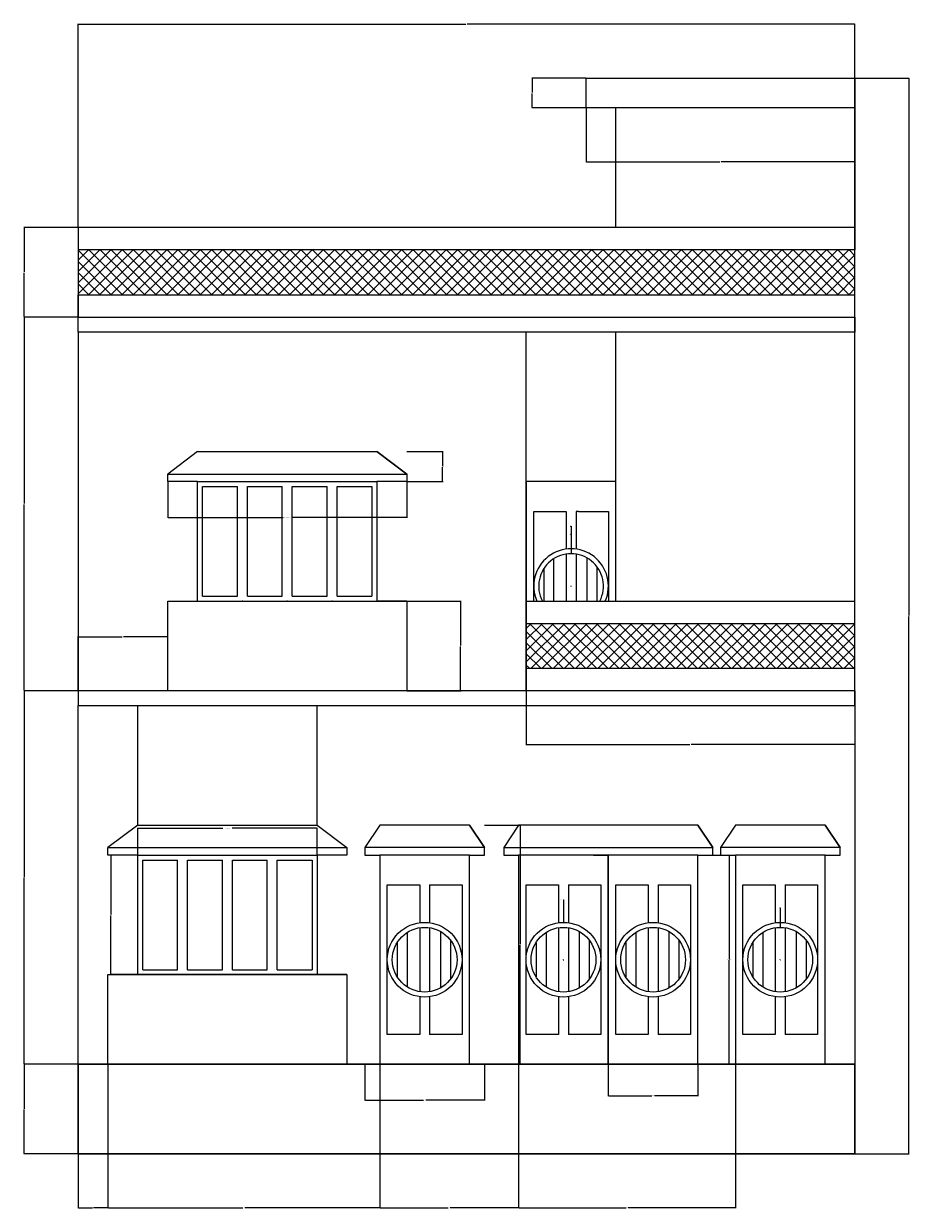
# Model space of a CAD drawing. Units: millimetres. Extents: x 1831 to 2754, y 1517 to 2450.
# Tile 3 of 4: x 1831 to 2186, y 1975 to 2450. Entities that reach past the tile are written whole.
import ezdxf

# ---------------------------------------------------------------- set-up
doc = ezdxf.new("R2010")
doc.units = ezdxf.units.MM
for name, color, linetype, lineweight in [('A-ANNO-DIMS', 2, 'Continuous', 18), ('A-DETL-REFP', 8, 'Continuous', 13), ('A-DOOR', 3, 'Continuous', 25), ('A-ELEV', 7, 'Continuous', 25), ('A-ELEV-BASE', 7, 'Continuous', 30), ('A-ELEV-PATT', 8, 'Continuous', 13), ('A-ELEV-SHAD', 7, 'Continuous', 18), ('A-GLAZ', 4, 'Continuous', 18), ('A-ROOF', 7, 'Continuous', 25)]:
    doc.layers.add(name, color=color, linetype=linetype, lineweight=lineweight)
doc.styles.get("Standard").update_dxf_attribs({"font": 'arial.ttf'})
doc.dimstyles.get("Standard").update_dxf_attribs({"dimtxt": 0.18, "dimasz": 0.18, "dimexe": 0.18, "dimexo": 0.0625, "dimgap": 0.09, "dimtad": 0, "dimtih": 1, "dimtoh": 1, "dimdec": 4, "dimzin": 0, "dimdsep": 46, "dimtxsty": 'Standard', "dimcen": 0.09, "dimadec": 0, "dimazin": 0, "dimtfac": 1, "dimtdec": 4, "dimtofl": 0, "dimtmove": 0, "dimatfit": 3, "dimfxl": 1, "dimtolj": 1, "dimtzin": 0, "dimarcsym": 0})

# ---------------------------------------------------------------- blocks, each defined once
blk = doc.blocks.new('DOOR-ELEV-SINGLE-HOODED')
for p, q in [((6, 96), (0, 87)), ((6, 96), (0, 87)), ((42, 96), (6, 96)), ((42, 96), (6, 96)), ((42, 96), (48, 87)), ((48, 87), (42, 96)), ((42, 96), (48, 87)), ((48, 87), (42, 96)), ((48, 87), (0, 87)), ((0, 87), (0, 84)), ((48, 87), (0, 87)), ((48, 84), (48, 87)), ((0, 84), (6, 84)), ((42, 84), (6, 84)), ((6, 84), (6, 0)), ((42, 84), (6, 84)), ((6, 84), (6, 0)), ((42, 0), (42, 84)), ((42, 84), (48, 84)), ((42, 0), (42, 84)), ((42, 84), (48, 84)), ((9, 72), (21, 72)), ((9, 12), (9, 72)), ((9, 72), (21, 72)), ((9, 12), (9, 72)), ((21, 72), (22, 72)), ((21, 72), (22, 72)), ((22, 72), (22, 56.87)), ((22, 72), (22, 56.87)), ((26, 72), (26, 56.87)), ((26, 72), (27, 72)), ((26, 72), (26, 56.87)), ((26, 72), (27, 72)), ((27, 72), (39, 72)), ((27, 72), (39, 72)), ((39, 72), (39, 12)), ((39, 72), (39, 12)), ((17, 52.95), (17, 31.05)), ((17, 52.95), (17, 31.05)), ((22, 54.85), (22, 29.15)), ((22, 54.85), (22, 29.15)), ((26, 54.85), (26, 29.15)), ((26, 54.85), (26, 29.15)), ((30.5, 30.74), (30.5, 53.26)), ((30.5, 30.74), (30.5, 53.26)), ((30.5, 30.74), (30.5, 53.26)), ((30.5, 30.74), (30.5, 53.26)), ((13, 48.93), (13, 35.07)), ((13, 48.93), (13, 35.07)), ((34.5, 34.34), (34.5, 49.66)), ((34.5, 34.34), (34.5, 49.66)), ((22, 27.13), (22, 12)), ((22, 27.13), (22, 12)), ((26, 27.13), (26, 12)), ((26, 27.13), (26, 12)), ((22, 12), (9, 12)), ((22, 12), (9, 12)), ((39, 12), (26, 12)), ((39, 12), (26, 12)), ((6, 0), (42, 0))]:
    blk.add_line(p, q)
for radius in [15, 15, 13, 13]:
    blk.add_circle((24, 42), radius)
blk = doc.blocks.new('DOOR-ELEV-ORNAMENTAL-LEAF')
for p, q in [((36, 84), (0, 84)), ((0, 84), (0, 0)), ((36, 0), (36, 84)), ((3, 72), (15, 72)), ((3, 12), (3, 72)), ((15, 72), (16, 72)), ((16, 72), (16, 56.87)), ((20, 72), (20, 56.87)), ((20, 72), (21, 72)), ((21, 72), (33, 72)), ((33, 72), (33, 12)), ((11, 52.95), (11, 31.05)), ((16, 54.85), (16, 29.15)), ((20, 54.85), (20, 29.15)), ((24.5, 30.74), (24.5, 53.26)), ((24.5, 30.74), (24.5, 53.26)), ((7, 48.93), (7, 35.07)), ((28.5, 34.34), (28.5, 49.66)), ((16, 27.13), (16, 12)), ((20, 27.13), (20, 12)), ((16, 12), (3, 12)), ((33, 12), (20, 12)), ((0, 0), (36, 0))]:
    blk.add_line(p, q)
for radius in [15, 13]:
    blk.add_circle((18, 42), radius)
blk = doc.blocks.new('WINDOW-ELEV-FOUR-LIGHT')
for p, q in [((0, 0), (0, 48)), ((0, 48), (72, 48)), ((72, 48), (72, 0)), ((2, 46), (16, 46)), ((2, 2), (2, 46)), ((16, 2), (16, 46)), ((20, 2), (20, 46)), ((20, 46), (34, 46)), ((34, 2), (34, 46)), ((38, 2), (38, 46)), ((38, 46), (52, 46)), ((52, 2), (52, 46)), ((56, 2), (56, 46)), ((56, 46), (70, 46)), ((70, 46), (70, 2)), ((0, 0), (72, 0)), ((2, 2), (16, 2)), ((20, 2), (34, 2)), ((38, 2), (52, 2)), ((56, 2), (70, 2))]:
    blk.add_line(p, q)
blk = doc.blocks.new('CANOPY-ELEV-WINDOW')
for p, q in [((12, 12), (0, 3)), ((12, 12), (84, 12)), ((84, 12), (96, 3)), ((0, 0), (0, 3)), ((0, 3), (96, 3)), ((12, 0), (0, 0)), ((96, 0), (84, 0)), ((96, 3), (96, 0))]:
    blk.add_line(p, q)
blk = doc.blocks.new('*D14')
at = {"layer": 'A-ANNO-DIMS', "color": 0, "lineweight": -2, "transparency": 16777216}
for p, q in [((2015.67, 2128.5), (2030.19, 2128.5)), ((2030.01, 2128.32), (2030.01, 2080.68)), ((2030.01, 2032.68), (2030.01, 2080.31)), ((2015.67, 2032.5), (2030.19, 2032.5))]:
    blk.add_line(p, q, dxfattribs=at)
at = {"layer": 'A-ANNO-DIMS', "color": 0, "transparency": 16777216}
for points in [[(2029.98, 2128.32), (2030.04, 2128.32), (2030.01, 2128.5)], [(2029.98, 2032.68), (2030.04, 2032.68), (2030.01, 2032.5)]]:
    blk.add_solid(points, dxfattribs=at)
at = {"layer": 'Defpoints', "color": 0, "transparency": 16777216}
for p in [(2015.61, 2128.5), (2030.01, 2128.5), (2015.61, 2032.5)]:
    blk.add_point(p, dxfattribs=at)
at = {"layer": 'A-ANNO-DIMS', "color": 0, "transparency": 16777216, "insert": (2030.01, 2080.5), "char_height": 0.18, "attachment_point": 5}
blk.add_mtext('\\A1;HOODED ENTRY 96 TYP.', dxfattribs=at)
blk = doc.blocks.new('*D15')
at = {"layer": 'A-ANNO-DIMS', "color": 0, "lineweight": -2, "transparency": 16777216}
for p, q in [((1967.61, 2032.43), (1967.61, 2017.92)), ((2015.61, 2032.43), (2015.61, 2017.92)), ((1967.79, 2018.1), (1991.08, 2018.1)), ((2015.43, 2018.1), (1992.14, 2018.1))]:
    blk.add_line(p, q, dxfattribs=at)
at = {"layer": 'A-ANNO-DIMS', "color": 0, "transparency": 16777216}
for points in [[(1967.79, 2018.13), (1967.79, 2018.07), (1967.61, 2018.1)], [(2015.43, 2018.13), (2015.43, 2018.07), (2015.61, 2018.1)]]:
    blk.add_solid(points, dxfattribs=at)
at = {"layer": 'Defpoints', "color": 0, "transparency": 16777216}
for p in [(1967.61, 2032.5), (2015.61, 2032.5), (2015.61, 2018.1)]:
    blk.add_point(p, dxfattribs=at)
at = {"layer": 'A-ANNO-DIMS', "color": 0, "transparency": 16777216, "insert": (1991.61, 2018.1), "char_height": 0.18, "attachment_point": 5}
blk.add_mtext('\\A1;48 TYP.', dxfattribs=at)
blk = doc.blocks.new('*D16')
at = {"layer": 'A-ANNO-DIMS', "color": 0, "lineweight": -2, "transparency": 16777216}
for p, q in [((2101.41, 2116.5), (2114.13, 2116.5)), ((2113.95, 2116.32), (2113.95, 2074.68)), ((2113.95, 2032.68), (2113.95, 2074.31)), ((2101.41, 2032.5), (2114.13, 2032.5))]:
    blk.add_line(p, q, dxfattribs=at)
at = {"layer": 'A-ANNO-DIMS', "color": 0, "transparency": 16777216}
for points in [[(2113.92, 2116.32), (2113.98, 2116.32), (2113.95, 2116.5)], [(2113.92, 2032.68), (2113.98, 2032.68), (2113.95, 2032.5)]]:
    blk.add_solid(points, dxfattribs=at)
at = {"layer": 'Defpoints', "color": 0, "transparency": 16777216}
for p in [(2101.35, 2116.5), (2113.95, 2116.5), (2101.35, 2032.5)]:
    blk.add_point(p, dxfattribs=at)
at = {"layer": 'A-ANNO-DIMS', "color": 0, "transparency": 16777216, "insert": (2113.95, 2074.5), "char_height": 0.18, "attachment_point": 5}
blk.add_mtext('\\A1;GATE LEAF 84 TYP.', dxfattribs=at)
blk = doc.blocks.new('*D17')
at = {"layer": 'A-ANNO-DIMS', "color": 0, "lineweight": -2, "transparency": 16777216}
for p, q in [((2065.35, 2032.43), (2065.35, 2019.72)), ((2101.35, 2032.43), (2101.35, 2019.72)), ((2065.53, 2019.9), (2082.82, 2019.9)), ((2101.17, 2019.9), (2083.88, 2019.9))]:
    blk.add_line(p, q, dxfattribs=at)
at = {"layer": 'A-ANNO-DIMS', "color": 0, "transparency": 16777216}
for points in [[(2065.53, 2019.93), (2065.53, 2019.87), (2065.35, 2019.9)], [(2101.17, 2019.93), (2101.17, 2019.87), (2101.35, 2019.9)]]:
    blk.add_solid(points, dxfattribs=at)
at = {"layer": 'Defpoints', "color": 0, "transparency": 16777216}
for p in [(2065.35, 2032.5), (2101.35, 2032.5), (2101.35, 2019.9)]:
    blk.add_point(p, dxfattribs=at)
at = {"layer": 'A-ANNO-DIMS', "color": 0, "transparency": 16777216, "insert": (2083.35, 2019.9), "char_height": 0.18, "attachment_point": 5}
blk.add_mtext('\\A1;36 TYP.', dxfattribs=at)
blk = doc.blocks.new('*D18')
at = {"layer": 'A-ANNO-DIMS', "color": 0, "lineweight": -2, "transparency": 16777216}
for p, q in [((1876.41, 2116.56), (1876.41, 2127.48)), ((1876.59, 2127.3), (1910.5, 2127.3)), ((1948.23, 2127.3), (1914.32, 2127.3)), ((1948.41, 2116.56), (1948.41, 2127.48))]:
    blk.add_line(p, q, dxfattribs=at)
at = {"layer": 'A-ANNO-DIMS', "color": 0, "transparency": 16777216}
for points in [[(1876.59, 2127.33), (1876.59, 2127.27), (1876.41, 2127.3)], [(1948.23, 2127.33), (1948.23, 2127.27), (1948.41, 2127.3)]]:
    blk.add_solid(points, dxfattribs=at)
at = {"layer": 'Defpoints', "color": 0, "transparency": 16777216}
for p in [(1948.41, 2127.3), (1876.41, 2116.5), (1948.41, 2116.5)]:
    blk.add_point(p, dxfattribs=at)
at = {"layer": 'A-ANNO-DIMS', "color": 0, "transparency": 16777216, "insert": (1912.41, 2127.3), "char_height": 0.18, "attachment_point": 5}
blk.add_mtext('\\A1;FOUR-LIGHT WINDOW 72 TYP.', dxfattribs=at)
blk = doc.blocks.new('*D19')
at = {"layer": 'A-ANNO-DIMS', "color": 0, "lineweight": -2, "transparency": 16777216}
for p, q in [((1876.35, 2116.5), (1865.43, 2116.5)), ((1865.61, 2116.32), (1865.61, 2092.68)), ((1865.61, 2068.68), (1865.61, 2092.31)), ((1876.35, 2068.5), (1865.43, 2068.5))]:
    blk.add_line(p, q, dxfattribs=at)
at = {"layer": 'A-ANNO-DIMS', "color": 0, "transparency": 16777216}
for points in [[(1865.58, 2116.32), (1865.64, 2116.32), (1865.61, 2116.5)], [(1865.58, 2068.68), (1865.64, 2068.68), (1865.61, 2068.5)]]:
    blk.add_solid(points, dxfattribs=at)
at = {"layer": 'Defpoints', "color": 0, "transparency": 16777216}
for p in [(1865.61, 2116.5), (1876.41, 2116.5), (1876.41, 2068.5)]:
    blk.add_point(p, dxfattribs=at)
at = {"layer": 'A-ANNO-DIMS', "color": 0, "transparency": 16777216, "insert": (1865.61, 2092.5), "char_height": 0.18, "attachment_point": 5}
blk.add_mtext('\\A1;48 TYP.', dxfattribs=at)
blk = doc.blocks.new('*D20')
at = {"layer": 'A-ANNO-DIMS', "color": 0, "lineweight": -2, "transparency": 16777216}
for p, q in [((1888.41, 2266.43), (1888.41, 2251.92)), ((1984.41, 2266.43), (1984.41, 2251.92)), ((1888.59, 2252.1), (1934.72, 2252.1)), ((1984.23, 2252.1), (1938.09, 2252.1))]:
    blk.add_line(p, q, dxfattribs=at)
at = {"layer": 'A-ANNO-DIMS', "color": 0, "transparency": 16777216}
for points in [[(1888.59, 2252.13), (1888.59, 2252.07), (1888.41, 2252.1)], [(1984.23, 2252.13), (1984.23, 2252.07), (1984.41, 2252.1)]]:
    blk.add_solid(points, dxfattribs=at)
at = {"layer": 'Defpoints', "color": 0, "transparency": 16777216}
for p in [(1888.41, 2266.5), (1984.41, 2266.5), (1984.41, 2252.1)]:
    blk.add_point(p, dxfattribs=at)
at = {"layer": 'A-ANNO-DIMS', "color": 0, "transparency": 16777216, "insert": (1936.41, 2252.1), "char_height": 0.18, "attachment_point": 5}
blk.add_mtext('\\A1;WINDOW CANOPY 96 TYP.', dxfattribs=at)
blk = doc.blocks.new('*D21')
at = {"layer": 'A-ANNO-DIMS', "color": 0, "lineweight": -2, "transparency": 16777216}
for p, q in [((1984.47, 2278.5), (1998.99, 2278.5)), ((1998.81, 2278.32), (1998.81, 2272.68)), ((1998.81, 2266.68), (1998.81, 2272.31)), ((1984.47, 2266.5), (1998.99, 2266.5))]:
    blk.add_line(p, q, dxfattribs=at)
at = {"layer": 'A-ANNO-DIMS', "color": 0, "transparency": 16777216}
for points in [[(1998.78, 2278.32), (1998.84, 2278.32), (1998.81, 2278.5)], [(1998.78, 2266.68), (1998.84, 2266.68), (1998.81, 2266.5)]]:
    blk.add_solid(points, dxfattribs=at)
at = {"layer": 'Defpoints', "color": 0, "transparency": 16777216}
for p in [(1984.41, 2278.5), (1998.81, 2278.5), (1984.41, 2266.5)]:
    blk.add_point(p, dxfattribs=at)
at = {"layer": 'A-ANNO-DIMS', "color": 0, "transparency": 16777216, "insert": (1998.81, 2272.5), "char_height": 0.18, "attachment_point": 5}
blk.add_mtext('\\A1;12 TYP.', dxfattribs=at)
blk = doc.blocks.new('*D45')
at = {"layer": 'A-ANNO-DIMS', "color": 0, "lineweight": -2, "transparency": 16777216}
for p, q in [((1852.41, 2368.56), (1852.41, 2450.31)), ((1852.59, 2450.13), (2008.12, 2450.13)), ((2164.23, 2450.13), (2008.7, 2450.13)), ((2164.41, 2428.56), (2164.41, 2450.31))]:
    blk.add_line(p, q, dxfattribs=at)
at = {"layer": 'A-ANNO-DIMS', "color": 0, "transparency": 16777216}
for points in [[(1852.59, 2450.16), (1852.59, 2450.1), (1852.41, 2450.13)], [(2164.23, 2450.16), (2164.23, 2450.1), (2164.41, 2450.13)]]:
    blk.add_solid(points, dxfattribs=at)
at = {"layer": 'Defpoints', "color": 0, "transparency": 16777216}
for p in [(2164.41, 2450.13), (2164.41, 2428.5), (1852.41, 2368.5)]:
    blk.add_point(p, dxfattribs=at)
at = {"layer": 'A-ANNO-DIMS', "color": 0, "transparency": 16777216, "insert": (2008.41, 2450.13), "char_height": 0.18, "attachment_point": 5}
blk.add_mtext('\\A1;312', dxfattribs=at)
blk = doc.blocks.new('*D46')
at = {"layer": 'A-ANNO-DIMS', "color": 0, "lineweight": -2, "transparency": 16777216}
for p, q in [((2164.47, 2428.5), (2186.22, 2428.5)), ((2186.04, 2428.32), (2186.04, 2212.68)), ((2186.04, 1996.68), (2186.04, 2212.31)), ((2164.47, 1996.5), (2186.22, 1996.5))]:
    blk.add_line(p, q, dxfattribs=at)
at = {"layer": 'A-ANNO-DIMS', "color": 0, "transparency": 16777216}
for points in [[(2186.01, 2428.32), (2186.07, 2428.32), (2186.04, 2428.5)], [(2186.01, 1996.68), (2186.07, 1996.68), (2186.04, 1996.5)]]:
    blk.add_solid(points, dxfattribs=at)
at = {"layer": 'Defpoints', "color": 0, "transparency": 16777216}
for p in [(2164.41, 2428.5), (2186.04, 2428.5), (2164.41, 1996.5)]:
    blk.add_point(p, dxfattribs=at)
at = {"layer": 'A-ANNO-DIMS', "color": 0, "transparency": 16777216, "insert": (2186.04, 2212.5), "char_height": 0.18, "attachment_point": 5}
blk.add_mtext('\\A1;432', dxfattribs=at)
blk = doc.blocks.new('*D47')
at = {"layer": 'A-ANNO-DIMS', "color": 0, "lineweight": -2, "transparency": 16777216}
for p, q in [((1852.35, 2032.5), (1830.6, 2032.5)), ((1830.78, 2032.32), (1830.78, 2014.68)), ((1830.78, 1996.68), (1830.78, 2014.31)), ((1852.35, 1996.5), (1830.6, 1996.5))]:
    blk.add_line(p, q, dxfattribs=at)
at = {"layer": 'A-ANNO-DIMS', "color": 0, "transparency": 16777216}
for points in [[(1830.75, 2032.32), (1830.81, 2032.32), (1830.78, 2032.5)], [(1830.75, 1996.68), (1830.81, 1996.68), (1830.78, 1996.5)]]:
    blk.add_solid(points, dxfattribs=at)
at = {"layer": 'Defpoints', "color": 0, "transparency": 16777216}
for p in [(1830.78, 2032.5), (1852.41, 2032.5), (1852.41, 1996.5)]:
    blk.add_point(p, dxfattribs=at)
at = {"layer": 'A-ANNO-DIMS', "color": 0, "transparency": 16777216, "insert": (1830.78, 2014.5), "char_height": 0.18, "attachment_point": 5}
blk.add_mtext('\\A1;36', dxfattribs=at)
blk = doc.blocks.new('*D48')
at = {"layer": 'A-ANNO-DIMS', "color": 0, "lineweight": -2, "transparency": 16777216}
for p, q in [((1852.35, 2182.5), (1830.6, 2182.5)), ((1830.78, 2182.32), (1830.78, 2107.68)), ((1830.78, 2032.68), (1830.78, 2107.31)), ((1852.35, 2032.5), (1830.6, 2032.5))]:
    blk.add_line(p, q, dxfattribs=at)
at = {"layer": 'A-ANNO-DIMS', "color": 0, "transparency": 16777216}
for points in [[(1830.75, 2182.32), (1830.81, 2182.32), (1830.78, 2182.5)], [(1830.75, 2032.68), (1830.81, 2032.68), (1830.78, 2032.5)]]:
    blk.add_solid(points, dxfattribs=at)
at = {"layer": 'Defpoints', "color": 0, "transparency": 16777216}
for p in [(1830.78, 2182.5), (1852.41, 2182.5), (1852.41, 2032.5)]:
    blk.add_point(p, dxfattribs=at)
at = {"layer": 'A-ANNO-DIMS', "color": 0, "transparency": 16777216, "insert": (1830.78, 2107.5), "char_height": 0.18, "attachment_point": 5}
blk.add_mtext('\\A1;150', dxfattribs=at)
blk = doc.blocks.new('*D49')
at = {"layer": 'A-ANNO-DIMS', "color": 0, "lineweight": -2, "transparency": 16777216}
for p, q in [((1852.35, 2332.5), (1830.6, 2332.5)), ((1830.78, 2332.32), (1830.78, 2257.68)), ((1830.78, 2182.68), (1830.78, 2257.31)), ((1852.35, 2182.5), (1830.6, 2182.5))]:
    blk.add_line(p, q, dxfattribs=at)
at = {"layer": 'A-ANNO-DIMS', "color": 0, "transparency": 16777216}
for points in [[(1830.75, 2332.32), (1830.81, 2332.32), (1830.78, 2332.5)], [(1830.75, 2182.68), (1830.81, 2182.68), (1830.78, 2182.5)]]:
    blk.add_solid(points, dxfattribs=at)
at = {"layer": 'Defpoints', "color": 0, "transparency": 16777216}
for p in [(1830.78, 2332.5), (1852.41, 2332.5), (1852.41, 2182.5)]:
    blk.add_point(p, dxfattribs=at)
at = {"layer": 'A-ANNO-DIMS', "color": 0, "transparency": 16777216, "insert": (1830.78, 2257.5), "char_height": 0.18, "attachment_point": 5}
blk.add_mtext('\\A1;150', dxfattribs=at)
blk = doc.blocks.new('*D50')
at = {"layer": 'A-ANNO-DIMS', "color": 0, "lineweight": -2, "transparency": 16777216}
for p, q in [((1852.35, 2368.5), (1830.6, 2368.5)), ((1830.78, 2368.32), (1830.78, 2350.68)), ((1830.78, 2332.68), (1830.78, 2350.31)), ((1852.35, 2332.5), (1830.6, 2332.5))]:
    blk.add_line(p, q, dxfattribs=at)
at = {"layer": 'A-ANNO-DIMS', "color": 0, "transparency": 16777216}
for points in [[(1830.75, 2368.32), (1830.81, 2368.32), (1830.78, 2368.5)], [(1830.75, 2332.68), (1830.81, 2332.68), (1830.78, 2332.5)]]:
    blk.add_solid(points, dxfattribs=at)
at = {"layer": 'Defpoints', "color": 0, "transparency": 16777216}
for p in [(1830.78, 2368.5), (1852.41, 2368.5), (1852.41, 2332.5)]:
    blk.add_point(p, dxfattribs=at)
at = {"layer": 'A-ANNO-DIMS', "color": 0, "transparency": 16777216, "insert": (1830.78, 2350.5), "char_height": 0.18, "attachment_point": 5}
blk.add_mtext('\\A1;36', dxfattribs=at)
blk = doc.blocks.new('*D51')
at = {"layer": 'A-ANNO-DIMS', "color": 0, "lineweight": -2, "transparency": 16777216}
for p, q in [((2056.41, 2416.43), (2056.41, 2394.69)), ((2164.41, 2416.43), (2164.41, 2394.69)), ((2056.59, 2394.87), (2110.13, 2394.87)), ((2164.23, 2394.87), (2110.69, 2394.87))]:
    blk.add_line(p, q, dxfattribs=at)
at = {"layer": 'A-ANNO-DIMS', "color": 0, "transparency": 16777216}
for points in [[(2056.59, 2394.9), (2056.59, 2394.84), (2056.41, 2394.87)], [(2164.23, 2394.9), (2164.23, 2394.84), (2164.41, 2394.87)]]:
    blk.add_solid(points, dxfattribs=at)
at = {"layer": 'Defpoints', "color": 0, "transparency": 16777216}
for p in [(2056.41, 2416.5), (2164.41, 2416.5), (2056.41, 2394.87)]:
    blk.add_point(p, dxfattribs=at)
at = {"layer": 'A-ANNO-DIMS', "color": 0, "transparency": 16777216, "insert": (2110.41, 2394.87), "char_height": 0.18, "attachment_point": 5}
blk.add_mtext('\\A1;108', dxfattribs=at)
blk = doc.blocks.new('*D52')
at = {"layer": 'A-ANNO-DIMS', "color": 0, "lineweight": -2, "transparency": 16777216}
for p, q in [((2056.35, 2428.5), (2034.6, 2428.5)), ((2034.78, 2428.32), (2034.78, 2422.68)), ((2034.78, 2416.68), (2034.78, 2422.31)), ((2056.35, 2416.5), (2034.6, 2416.5))]:
    blk.add_line(p, q, dxfattribs=at)
at = {"layer": 'A-ANNO-DIMS', "color": 0, "transparency": 16777216}
for points in [[(2034.75, 2428.32), (2034.81, 2428.32), (2034.78, 2428.5)], [(2034.75, 2416.68), (2034.81, 2416.68), (2034.78, 2416.5)]]:
    blk.add_solid(points, dxfattribs=at)
at = {"layer": 'Defpoints', "color": 0, "transparency": 16777216}
for p in [(2034.78, 2428.5), (2056.41, 2428.5), (2056.41, 2416.5)]:
    blk.add_point(p, dxfattribs=at)
at = {"layer": 'A-ANNO-DIMS', "color": 0, "transparency": 16777216, "insert": (2034.78, 2422.5), "char_height": 0.18, "attachment_point": 5}
blk.add_mtext('\\A1;12', dxfattribs=at)
blk = doc.blocks.new('*D53')
at = {"layer": 'A-ANNO-DIMS', "color": 0, "lineweight": -2, "transparency": 16777216}
for p, q in [((2032.41, 2182.43), (2032.41, 2160.69)), ((2164.41, 2182.43), (2164.41, 2160.69)), ((2032.59, 2160.87), (2098.13, 2160.87)), ((2164.23, 2160.87), (2098.69, 2160.87))]:
    blk.add_line(p, q, dxfattribs=at)
at = {"layer": 'A-ANNO-DIMS', "color": 0, "transparency": 16777216}
for points in [[(2032.59, 2160.9), (2032.59, 2160.84), (2032.41, 2160.87)], [(2164.23, 2160.9), (2164.23, 2160.84), (2164.41, 2160.87)]]:
    blk.add_solid(points, dxfattribs=at)
at = {"layer": 'Defpoints', "color": 0, "transparency": 16777216}
for p in [(2032.41, 2182.5), (2164.41, 2182.5), (2032.41, 2160.87)]:
    blk.add_point(p, dxfattribs=at)
at = {"layer": 'A-ANNO-DIMS', "color": 0, "transparency": 16777216, "insert": (2098.41, 2160.87), "char_height": 0.18, "attachment_point": 5}
blk.add_mtext('\\A1;132', dxfattribs=at)
blk = doc.blocks.new('*D54')
at = {"layer": 'A-ANNO-DIMS', "color": 0, "lineweight": -2, "transparency": 16777216}
for p, q in [((1984.47, 2218.5), (2006.22, 2218.5)), ((2006.04, 2218.32), (2006.04, 2200.68)), ((2006.04, 2182.68), (2006.04, 2200.31)), ((1984.47, 2182.5), (2006.22, 2182.5))]:
    blk.add_line(p, q, dxfattribs=at)
at = {"layer": 'A-ANNO-DIMS', "color": 0, "transparency": 16777216}
for points in [[(2006.01, 2218.32), (2006.07, 2218.32), (2006.04, 2218.5)], [(2006.01, 2182.68), (2006.07, 2182.68), (2006.04, 2182.5)]]:
    blk.add_solid(points, dxfattribs=at)
at = {"layer": 'Defpoints', "color": 0, "transparency": 16777216}
for p in [(1984.41, 2218.5), (1984.41, 2182.5), (2006.04, 2182.5)]:
    blk.add_point(p, dxfattribs=at)
at = {"layer": 'A-ANNO-DIMS', "color": 0, "transparency": 16777216, "insert": (2006.04, 2200.5), "char_height": 0.18, "attachment_point": 5}
blk.add_mtext('\\A1;36', dxfattribs=at)
blk = doc.blocks.new('*D55')
at = {"layer": 'A-ANNO-DIMS', "color": 0, "lineweight": -2, "transparency": 16777216}
for p, q in [((1852.41, 2032.43), (1852.41, 1974.69)), ((1864.41, 2032.43), (1864.41, 1974.69)), ((1852.59, 1974.87), (1858.2, 1974.87)), ((1864.23, 1974.87), (1858.62, 1974.87))]:
    blk.add_line(p, q, dxfattribs=at)
at = {"layer": 'A-ANNO-DIMS', "color": 0, "transparency": 16777216}
for points in [[(1852.59, 1974.9), (1852.59, 1974.84), (1852.41, 1974.87)], [(1864.23, 1974.9), (1864.23, 1974.84), (1864.41, 1974.87)]]:
    blk.add_solid(points, dxfattribs=at)
at = {"layer": 'Defpoints', "color": 0, "transparency": 16777216}
for p in [(1852.41, 2032.5), (1864.41, 2032.5), (1864.41, 1974.87)]:
    blk.add_point(p, dxfattribs=at)
at = {"layer": 'A-ANNO-DIMS', "color": 0, "transparency": 16777216, "insert": (1858.41, 1974.87), "char_height": 0.18, "attachment_point": 5}
blk.add_mtext('\\A1;12', dxfattribs=at)
blk = doc.blocks.new('*D56')
at = {"layer": 'A-ANNO-DIMS', "color": 0, "lineweight": -2, "transparency": 16777216}
for p, q in [((1864.41, 2032.43), (1864.41, 1974.69)), ((1973.61, 2032.43), (1973.61, 1974.69)), ((1864.59, 1974.87), (1918.62, 1974.87)), ((1973.43, 1974.87), (1919.39, 1974.87))]:
    blk.add_line(p, q, dxfattribs=at)
at = {"layer": 'A-ANNO-DIMS', "color": 0, "transparency": 16777216}
for points in [[(1864.59, 1974.9), (1864.59, 1974.84), (1864.41, 1974.87)], [(1973.43, 1974.9), (1973.43, 1974.84), (1973.61, 1974.87)]]:
    blk.add_solid(points, dxfattribs=at)
at = {"layer": 'Defpoints', "color": 0, "transparency": 16777216}
for p in [(1864.41, 2032.5), (1973.61, 2032.5), (1973.61, 1974.87)]:
    blk.add_point(p, dxfattribs=at)
at = {"layer": 'A-ANNO-DIMS', "color": 0, "transparency": 16777216, "insert": (1919.01, 1974.87), "char_height": 0.18, "attachment_point": 5}
blk.add_mtext('\\A1;109.2', dxfattribs=at)
blk = doc.blocks.new('*D57')
at = {"layer": 'A-ANNO-DIMS', "color": 0, "lineweight": -2, "transparency": 16777216}
for p, q in [((1973.61, 2032.43), (1973.61, 1974.69)), ((2029.35, 2032.43), (2029.35, 1974.69)), ((1973.79, 1974.87), (2001.09, 1974.87)), ((2029.17, 1974.87), (2001.87, 1974.87))]:
    blk.add_line(p, q, dxfattribs=at)
at = {"layer": 'A-ANNO-DIMS', "color": 0, "transparency": 16777216}
for points in [[(1973.79, 1974.9), (1973.79, 1974.84), (1973.61, 1974.87)], [(2029.17, 1974.9), (2029.17, 1974.84), (2029.35, 1974.87)]]:
    blk.add_solid(points, dxfattribs=at)
at = {"layer": 'Defpoints', "color": 0, "transparency": 16777216}
for p in [(1973.61, 2032.5), (2029.35, 2032.5), (2029.35, 1974.87)]:
    blk.add_point(p, dxfattribs=at)
at = {"layer": 'A-ANNO-DIMS', "color": 0, "transparency": 16777216, "insert": (2001.48, 1974.87), "char_height": 0.18, "attachment_point": 5}
blk.add_mtext('\\A1;55.74', dxfattribs=at)
blk = doc.blocks.new('*D58')
at = {"layer": 'A-ANNO-DIMS', "color": 0, "lineweight": -2, "transparency": 16777216}
for p, q in [((2029.35, 2032.43), (2029.35, 1974.69)), ((2116.41, 2032.43), (2116.41, 1974.69)), ((2029.53, 1974.87), (2072.49, 1974.87)), ((2116.23, 1974.87), (2073.27, 1974.87))]:
    blk.add_line(p, q, dxfattribs=at)
at = {"layer": 'A-ANNO-DIMS', "color": 0, "transparency": 16777216}
for points in [[(2029.53, 1974.9), (2029.53, 1974.84), (2029.35, 1974.87)], [(2116.23, 1974.9), (2116.23, 1974.84), (2116.41, 1974.87)]]:
    blk.add_solid(points, dxfattribs=at)
at = {"layer": 'Defpoints', "color": 0, "transparency": 16777216}
for p in [(2029.35, 2032.5), (2116.41, 2032.5), (2116.41, 1974.87)]:
    blk.add_point(p, dxfattribs=at)
at = {"layer": 'A-ANNO-DIMS', "color": 0, "transparency": 16777216, "insert": (2072.88, 1974.87), "char_height": 0.18, "attachment_point": 5}
blk.add_mtext('\\A1;87.06', dxfattribs=at)
blk = doc.blocks.new('*D59')
at = {"layer": 'A-ANNO-DIMS', "color": 0, "lineweight": -2, "transparency": 16777216}
for p, q in [((1852.41, 2182.56), (1852.41, 2204.31)), ((1852.59, 2204.13), (1870.19, 2204.13)), ((1888.23, 2204.13), (1870.63, 2204.13)), ((1888.41, 2182.56), (1888.41, 2204.31))]:
    blk.add_line(p, q, dxfattribs=at)
at = {"layer": 'A-ANNO-DIMS', "color": 0, "transparency": 16777216}
for points in [[(1852.59, 2204.16), (1852.59, 2204.1), (1852.41, 2204.13)], [(1888.23, 2204.16), (1888.23, 2204.1), (1888.41, 2204.13)]]:
    blk.add_solid(points, dxfattribs=at)
at = {"layer": 'Defpoints', "color": 0, "transparency": 16777216}
for p in [(1888.41, 2204.13), (1852.41, 2182.5), (1888.41, 2182.5)]:
    blk.add_point(p, dxfattribs=at)
at = {"layer": 'A-ANNO-DIMS', "color": 0, "transparency": 16777216, "insert": (1870.41, 2204.13), "char_height": 0.18, "attachment_point": 5}
blk.add_mtext('\\A1;36', dxfattribs=at)
blk = doc.blocks.new('*D72')
at = {"layer": 'A-ANNO-DIMS', "color": 0, "lineweight": -2, "transparency": 16777216}
for p, q in [((2047.17, 2098.5), (2047.35, 2098.5)), ((2047.35, 2098.5), (2047.35, 2089.68)), ((2047.26, 2074.5), (2047.44, 2074.5)), ((2047.35, 2074.41), (2047.35, 2074.59))]:
    blk.add_line(p, q, dxfattribs=at)
at = {"layer": 'A-ANNO-DIMS', "color": 0, "transparency": 16777216}
blk.add_solid([(2047.38, 2089.68), (2047.32, 2089.68), (2047.35, 2089.5)], dxfattribs=at)
at = {"layer": 'Defpoints', "color": 0, "transparency": 16777216}
for p in [(2047.35, 2089.5), (2047.35, 2059.5)]:
    blk.add_point(p, dxfattribs=at)
at = {"layer": 'A-ANNO-DIMS', "color": 0, "transparency": 16777216, "insert": (2046.66, 2098.5), "char_height": 0.18, "attachment_point": 5}
blk.add_mtext('\\A1;4X ∅30', dxfattribs=at)
blk = doc.blocks.new('*D73')
at = {"layer": 'A-ANNO-DIMS', "color": 0, "lineweight": -2, "transparency": 16777216}
for p, q in [((2134.23, 2095.3), (2134.41, 2095.3)), ((2134.41, 2095.3), (2134.41, 2087.68)), ((2134.32, 2074.5), (2134.5, 2074.5)), ((2134.41, 2074.41), (2134.41, 2074.59))]:
    blk.add_line(p, q, dxfattribs=at)
at = {"layer": 'A-ANNO-DIMS', "color": 0, "transparency": 16777216}
blk.add_solid([(2134.44, 2087.68), (2134.38, 2087.68), (2134.41, 2087.5)], dxfattribs=at)
at = {"layer": 'Defpoints', "color": 0, "transparency": 16777216}
for p in [(2134.41, 2087.5), (2134.41, 2061.5)]:
    blk.add_point(p, dxfattribs=at)
at = {"layer": 'A-ANNO-DIMS', "color": 0, "transparency": 16777216, "insert": (2133.72, 2095.3), "char_height": 0.18, "attachment_point": 5}
blk.add_mtext('\\A1;4X ∅26', dxfattribs=at)
blk = doc.blocks.new('*D74')
at = {"layer": 'A-ANNO-DIMS', "color": 0, "lineweight": -2, "transparency": 16777216}
for p, q in [((2050.23, 2248.5), (2050.41, 2248.5)), ((2050.41, 2248.5), (2050.41, 2239.68)), ((2050.32, 2224.5), (2050.5, 2224.5)), ((2050.41, 2224.41), (2050.41, 2224.59))]:
    blk.add_line(p, q, dxfattribs=at)
at = {"layer": 'A-ANNO-DIMS', "color": 0, "transparency": 16777216}
blk.add_solid([(2050.44, 2239.68), (2050.38, 2239.68), (2050.41, 2239.5)], dxfattribs=at)
at = {"layer": 'Defpoints', "color": 0, "transparency": 16777216}
for p in [(2050.41, 2239.5), (2050.41, 2224.5)]:
    blk.add_point(p, dxfattribs=at)
at = {"layer": 'A-ANNO-DIMS', "color": 0, "transparency": 16777216, "insert": (2049.92, 2248.5), "char_height": 0.18, "attachment_point": 5}
blk.add_mtext('\\A1;R15', dxfattribs=at)
blk = doc.blocks.new('*D75')
at = {"layer": 'A-ANNO-DIMS', "color": 0, "lineweight": -2, "transparency": 16777216}
for p, q in [((2050.23, 2245.3), (2050.41, 2245.3)), ((2050.41, 2245.3), (2050.41, 2237.68)), ((2050.32, 2224.5), (2050.5, 2224.5)), ((2050.41, 2224.41), (2050.41, 2224.59))]:
    blk.add_line(p, q, dxfattribs=at)
at = {"layer": 'A-ANNO-DIMS', "color": 0, "transparency": 16777216}
blk.add_solid([(2050.44, 2237.68), (2050.38, 2237.68), (2050.41, 2237.5)], dxfattribs=at)
at = {"layer": 'Defpoints', "color": 0, "transparency": 16777216}
for p in [(2050.41, 2237.5), (2050.41, 2224.5)]:
    blk.add_point(p, dxfattribs=at)
at = {"layer": 'A-ANNO-DIMS', "color": 0, "transparency": 16777216, "insert": (2049.92, 2245.3), "char_height": 0.18, "attachment_point": 5}
blk.add_mtext('\\A1;R13', dxfattribs=at)

msp = doc.modelspace()

# ---------------------------------------------------------------- hatches: boundary and pattern name
at = {"layer": 'A-ELEV-PATT'}
h = msp.add_hatch(dxfattribs=at)
h.set_pattern_fill('ANSI37', color=256)
h.paths.add_polyline_path([(2164.409, 2359.495), (1852.409, 2359.495), (1852.409, 2341.495), (2164.409, 2341.495)])
h = msp.add_hatch(dxfattribs=at)
h.set_pattern_fill('ANSI37', color=256)
h.paths.add_polyline_path([(2164.409, 2209.495), (2032.409, 2209.495), (2032.409, 2191.495), (2164.409, 2191.495)])

# ---------------------------------------------------------------- linework, layer by layer
at = {"layer": 'A-DETL-REFP'}
for p in [(1918.409, 2218.495), (1936.409, 2218.495), (1954.409, 2218.495), (1894.409, 2068.495), (1912.409, 2068.495), (1930.409, 2068.495)]:
    msp.add_point(p, dxfattribs=at)
at = {"layer": 'A-DOOR'}
for p, q in [((2068.409, 2266.495), (2032.409, 2266.495)), ((2032.409, 2266.495), (2032.409, 2182.495)), ((2068.409, 2266.495), (2032.409, 2266.495)), ((2032.409, 2266.495), (2032.409, 2182.495)), ((2068.409, 2218.495), (2068.409, 2266.495)), ((2068.409, 2218.495), (2068.409, 2266.495)), ((2035.409, 2254.495), (2047.409, 2254.495)), ((2035.409, 2218.495), (2035.409, 2254.495)), ((2035.409, 2254.495), (2047.409, 2254.495)), ((2035.409, 2218.495), (2035.409, 2254.495)), ((2047.409, 2254.495), (2048.409, 2254.495)), ((2047.409, 2254.495), (2048.409, 2254.495)), ((2048.409, 2254.495), (2048.409, 2239.361)), ((2048.409, 2254.495), (2048.409, 2239.361)), ((2052.409, 2254.495), (2052.409, 2239.361)), ((2052.409, 2254.495), (2052.409, 2239.361)), ((2053.409, 2254.495), (2052.409, 2254.495)), ((2053.409, 2254.495), (2065.409, 2254.495)), ((2065.409, 2254.495), (2065.409, 2218.495)), ((2065.409, 2254.495), (2065.409, 2218.495)), ((2043.409, 2235.45), (2043.409, 2218.495)), ((2043.409, 2235.45), (2043.409, 2218.495)), ((2048.409, 2237.34), (2048.409, 2218.495)), ((2048.409, 2237.34), (2048.409, 2218.495)), ((2052.409, 2237.34), (2052.409, 2218.495)), ((2052.409, 2237.34), (2052.409, 2218.495)), ((2056.909, 2218.495), (2056.909, 2235.753)), ((2056.909, 2218.495), (2056.909, 2235.753)), ((2056.909, 2218.495), (2056.909, 2235.753)), ((2056.909, 2218.495), (2056.909, 2235.753)), ((2039.409, 2231.423), (2039.409, 2218.495)), ((2039.409, 2231.423), (2039.409, 2218.495)), ((2060.909, 2218.495), (2060.909, 2232.16)), ((2060.909, 2218.495), (2060.909, 2232.16)), ((2116.409, 2032.495), (2152.409, 2032.495))]:
    msp.add_line(p, q, dxfattribs=at)
for radius, start, end in [(15, 336.42182, 203.57818), (15, 336.42182, 203.57818), (13, 332.51357, 207.48643), (13, 332.51357, 207.48643)]:
    msp.add_arc((2050.409, 2224.495), radius, start, end, dxfattribs=at)
at = {"layer": 'A-ELEV'}
for p, q in [((2164.409, 2326.495), (1852.409, 2326.495)), ((1852.409, 2326.495), (1852.409, 2182.495)), ((2032.409, 2182.495), (2032.409, 2326.495)), ((2068.409, 2266.495), (2068.409, 2326.495)), ((2164.409, 2182.495), (2164.409, 2326.495)), ((1888.409, 2182.495), (1888.409, 2218.495)), ((1888.409, 2218.495), (1984.409, 2218.495)), ((1888.409, 2218.495), (1900.409, 2218.495)), ((1984.409, 2218.495), (1972.409, 2218.495)), ((1984.409, 2218.495), (1984.409, 2182.495)), ((2032.409, 2218.495), (2164.409, 2218.495)), ((2032.409, 2209.495), (2164.409, 2209.495)), ((2032.409, 2191.495), (2164.409, 2191.495)), ((2164.409, 2182.495), (1852.409, 2182.495)), ((1852.409, 2182.495), (1852.409, 2176.495)), ((2164.409, 2182.495), (2032.409, 2182.495)), ((2164.409, 2176.495), (2164.409, 2182.495)), ((1852.409, 2176.495), (2164.409, 2176.495)), ((1852.409, 2032.495), (1852.409, 2176.495)), ((1852.409, 2176.495), (2164.409, 2176.495)), ((1852.409, 2176.495), (1882.409, 2176.495)), ((1876.409, 2128.495), (1876.409, 2176.495)), ((1882.409, 2176.495), (1888.409, 2176.495)), ((1948.409, 2128.495), (1948.409, 2176.495)), ((2164.409, 2176.495), (2164.409, 2032.495)), ((1864.409, 2032.495), (1864.409, 2068.495)), ((1864.409, 2068.495), (1924.409, 2068.495)), ((1864.409, 2068.495), (1960.409, 2068.495)), ((1912.409, 2068.495), (1876.409, 2068.495)), ((1960.409, 2068.495), (1912.409, 2068.495)), ((1924.409, 2068.495), (1936.409, 2068.495)), ((1936.409, 2068.495), (1960.409, 2068.495)), ((1960.409, 2068.495), (1960.409, 2032.495)), ((2116.409, 2032.495), (2104.409, 2032.495)), ((2104.409, 2032.495), (2104.409, 2032.495)), ((2164.409, 2032.495), (2152.409, 2032.495))]:
    msp.add_line(p, q, dxfattribs=at)
at = {"layer": 'A-ELEV-BASE'}
for p, q in [((1852.409, 1996.495), (1852.409, 2032.495)), ((1852.409, 2032.495), (1912.409, 2032.495)), ((1852.409, 2032.495), (1864.409, 2032.495)), ((2164.409, 2032.495), (1864.409, 2032.495)), ((2164.409, 1996.495), (2164.409, 2032.495)), ((1912.409, 1996.495), (1852.409, 1996.495)), ((1864.409, 1996.495), (2164.409, 1996.495))]:
    msp.add_line(p, q, dxfattribs=at)
at = {"layer": 'A-ELEV-SHAD'}
for p, q in [((1984.409, 2269.495), (1972.409, 2278.495)), ((2029.35, 2128.495), (2023.35, 2119.495)), ((2065.35, 2128.495), (2029.35, 2128.495)), ((2101.35, 2128.495), (2065.35, 2128.495)), ((2101.35, 2128.495), (2107.35, 2119.495)), ((2107.35, 2119.495), (2101.35, 2128.495)), ((2023.35, 2119.495), (2023.35, 2116.495)), ((2023.35, 2119.495), (2107.35, 2119.495)), ((2107.35, 2116.495), (2107.35, 2119.495)), ((2023.35, 2116.495), (2029.35, 2116.495)), ((2059.35, 2116.495), (2065.35, 2116.495)), ((2101.35, 2116.495), (2107.35, 2116.495)), ((2110.409, 2116.495), (2116.409, 2116.495))]:
    msp.add_line(p, q, dxfattribs=at)
at = {"layer": 'A-ROOF'}
for p, q in [((2056.409, 2416.495), (2056.409, 2428.495)), ((2056.409, 2428.495), (2164.409, 2428.495)), ((2164.409, 2428.495), (2164.409, 2368.495)), ((2164.409, 2368.495), (2164.409, 2428.495)), ((2164.409, 2428.495), (2164.409, 2416.495)), ((2068.409, 2416.495), (2056.409, 2416.495)), ((2068.409, 2368.495), (2068.409, 2416.495)), ((2164.409, 2416.495), (2068.409, 2416.495)), ((2164.409, 2368.495), (1852.409, 2368.495)), ((1852.409, 2368.495), (1852.409, 2332.495)), ((2164.409, 2332.495), (2164.409, 2368.495)), ((2164.409, 2341.495), (2164.409, 2368.495)), ((2164.409, 2368.495), (2164.409, 2359.495)), ((2164.409, 2359.495), (1852.409, 2359.495)), ((1852.409, 2332.495), (1852.409, 2341.495)), ((1852.409, 2341.495), (2164.409, 2341.495)), ((1852.409, 2326.495), (1852.409, 2332.495)), ((1852.409, 2332.495), (2164.409, 2332.495)), ((2164.409, 2332.495), (2164.409, 2326.495)), ((2164.409, 2326.495), (2164.409, 2332.495))]:
    msp.add_line(p, q, dxfattribs=at)

# ---------------------------------------------------------------- block references
at = {"layer": 'A-DOOR'}
for name, p in [('DOOR-ELEV-SINGLE-HOODED', (1967.607, 2032.495)), ('DOOR-ELEV-SINGLE-HOODED', (2110.409, 2032.495)), ('DOOR-ELEV-ORNAMENTAL-LEAF', (2029.35, 2032.495)), ('DOOR-ELEV-ORNAMENTAL-LEAF', (2065.35, 2032.495))]:
    msp.add_blockref(name, p, dxfattribs=at)
at = {"layer": 'A-ELEV-SHAD'}
for p in [(1888.409, 2266.495), (1864.409, 2116.495)]:
    msp.add_blockref('CANOPY-ELEV-WINDOW', p, dxfattribs=at)
at = {"layer": 'A-GLAZ'}
for p in [(1900.409, 2218.495), (1876.409, 2068.495)]:
    msp.add_blockref('WINDOW-ELEV-FOUR-LIGHT', p, dxfattribs=at)

# ---------------------------------------------------------------- dimensions: what is measured, and where the dimension line sits
at = {"layer": 'A-ANNO-DIMS'}
for base, p1, p2, override, picture, middle in [((2164.409, 2450.125), (1852.409, 2368.495), (2164.409, 2428.495), {"dimdec": 0, "dimlfac": 1, "dimrnd": 0, "dimzin": 0, "dimdsep": 46, "dimlunit": 2}, '*D45', (2008.409, 2450.125)), ((1888.409, 2204.125), (1852.409, 2182.495), (1888.409, 2182.495), {"dimdec": 0, "dimlfac": 1, "dimrnd": 0, "dimzin": 0, "dimdsep": 46, "dimlunit": 2}, '*D59', (1870.409, 2204.125)), ((1864.409, 1974.865), (1852.409, 2032.495), (1864.409, 2032.495), {"dimdec": 0, "dimlfac": 1, "dimrnd": 0, "dimzin": 0, "dimdsep": 46, "dimlunit": 2}, '*D55', (1858.409, 1974.865)), ((1973.607, 1974.865), (1864.409, 2032.495), (1973.607, 2032.495), {"dimdec": 1, "dimlfac": 1, "dimrnd": 0, "dimzin": 0, "dimdsep": 46, "dimlunit": 2}, '*D56', (1919.008, 1974.865)), ((2029.35, 1974.865), (1973.607, 2032.495), (2029.35, 2032.495), {"dimdec": 2, "dimlfac": 1, "dimrnd": 0, "dimzin": 0, "dimdsep": 46, "dimlunit": 2}, '*D57', (2001.479, 1974.865)), ((2116.409, 1974.865), (2029.35, 2032.495), (2116.409, 2032.495), {"dimdec": 2, "dimlfac": 1, "dimrnd": 0, "dimzin": 0, "dimdsep": 46, "dimlunit": 2}, '*D58', (2072.88, 1974.865))]:
    dim = msp.add_linear_dim(base=base, p1=p1, p2=p2, dimstyle='Standard', override=override, dxfattribs=at)
    dim.commit()
    dim.dimension.update_dxf_attribs({"geometry": picture, "text_midpoint": middle})
for base, p1, p2, angle, picture, middle in [((2034.779, 2428.495), (2056.409, 2416.495), (2056.409, 2428.495), 90, '*D52', (2034.779, 2422.495)), ((2186.039, 2428.495), (2164.409, 1996.495), (2164.409, 2428.495), 90, '*D46', (2186.039, 2212.495)), ((2056.409, 2394.865), (2164.409, 2416.495), (2056.409, 2416.495), 180, '*D51', (2110.409, 2394.865)), ((1830.779, 2368.495), (1852.409, 2332.495), (1852.409, 2368.495), 90, '*D50', (1830.779, 2350.495)), ((1830.779, 2332.495), (1852.409, 2182.495), (1852.409, 2332.495), 90, '*D49', (1830.779, 2257.495)), ((2006.039, 2182.495), (1984.409, 2218.495), (1984.409, 2182.495), 270, '*D54', (2006.039, 2200.495)), ((1830.779, 2182.495), (1852.409, 2032.495), (1852.409, 2182.495), 90, '*D48', (1830.779, 2107.495)), ((2032.409, 2160.865), (2164.409, 2182.495), (2032.409, 2182.495), 180, '*D53', (2098.409, 2160.865)), ((1830.779, 2032.495), (1852.409, 1996.495), (1852.409, 2032.495), 90, '*D47', (1830.779, 2014.495))]:
    dim = msp.add_linear_dim(base=base, p1=p1, p2=p2, angle=angle, dimstyle='Standard', override={"dimdec": 0, "dimlfac": 1, "dimrnd": 0, "dimzin": 0, "dimdsep": 46, "dimlunit": 2}, dxfattribs=at)
    dim.commit()
    dim.dimension.update_dxf_attribs({"geometry": picture, "text_midpoint": middle})
for base, p1, p2, text, picture, middle in [((1998.809, 2278.495), (1984.409, 2266.495), (1984.409, 2278.495), '<> TYP.', '*D21', (1998.809, 2272.495)), ((2030.007, 2128.495), (2015.607, 2032.495), (2015.607, 2128.495), 'HOODED ENTRY <> TYP.', '*D14', (2030.007, 2080.495)), ((1865.609, 2116.495), (1876.409, 2068.495), (1876.409, 2116.495), '<> TYP.', '*D19', (1865.609, 2092.495)), ((2113.95, 2116.495), (2101.35, 2032.495), (2101.35, 2116.495), 'GATE LEAF <> TYP.', '*D16', (2113.95, 2074.495))]:
    dim = msp.add_linear_dim(base=base, p1=p1, p2=p2, angle=90, text=text, dimstyle='Standard', override={"dimdec": 0, "dimlfac": 1, "dimrnd": 0, "dimzin": 0, "dimdsep": 46, "dimlunit": 2}, dxfattribs=at)
    dim.commit()
    dim.dimension.update_dxf_attribs({"geometry": picture, "text_midpoint": middle})
for base, p1, p2, text, picture, middle in [((1984.409, 2252.095), (1888.409, 2266.495), (1984.409, 2266.495), 'WINDOW CANOPY <> TYP.', '*D20', (1936.409, 2252.095)), ((1948.409, 2127.295), (1876.409, 2116.495), (1948.409, 2116.495), 'FOUR-LIGHT WINDOW <> TYP.', '*D18', (1912.409, 2127.295)), ((2015.607, 2018.095), (1967.607, 2032.495), (2015.607, 2032.495), '<> TYP.', '*D15', (1991.607, 2018.095)), ((2101.35, 2019.895), (2065.35, 2032.495), (2101.35, 2032.495), '<> TYP.', '*D17', (2083.35, 2019.895))]:
    dim = msp.add_linear_dim(base=base, p1=p1, p2=p2, text=text, dimstyle='Standard', override={"dimdec": 0, "dimlfac": 1, "dimrnd": 0, "dimzin": 0, "dimdsep": 46, "dimlunit": 2}, dxfattribs=at)
    dim.commit()
    dim.dimension.update_dxf_attribs({"geometry": picture, "text_midpoint": middle})
for mpoint, picture, middle in [((2050.409, 2239.495), '*D74', (2049.923, 2248.495)), ((2050.409, 2237.495), '*D75', (2049.924, 2245.295))]:
    dim = msp.add_radius_dim(center=(2050.409, 2224.495), mpoint=mpoint, dimstyle='Standard', override={"dimdec": 0, "dimlfac": 1, "dimrnd": 0, "dimzin": 0, "dimdsep": 46, "dimlunit": 2}, dxfattribs=at)
    dim.commit()
    dim.dimension.update_dxf_attribs({"geometry": picture, "text_midpoint": middle, "dimtype": 164})
for p1, p2, picture, middle in [((2047.351, 2059.495), (2047.35, 2089.495), '*D72', (2046.661, 2098.495)), ((2134.409, 2061.495), (2134.409, 2087.495), '*D73', (2133.72, 2095.295))]:
    dim = msp.add_diameter_dim_2p(p1=p1, p2=p2, text='4X <>', dimstyle='Standard', override={"dimdec": 0, "dimlfac": 1, "dimrnd": 0, "dimzin": 0, "dimdsep": 46, "dimlunit": 2}, dxfattribs=at)
    dim.commit()
    dim.dimension.update_dxf_attribs({"geometry": picture, "text_midpoint": middle, "dimtype": 163})

doc.saveas('drawing.dxf')
